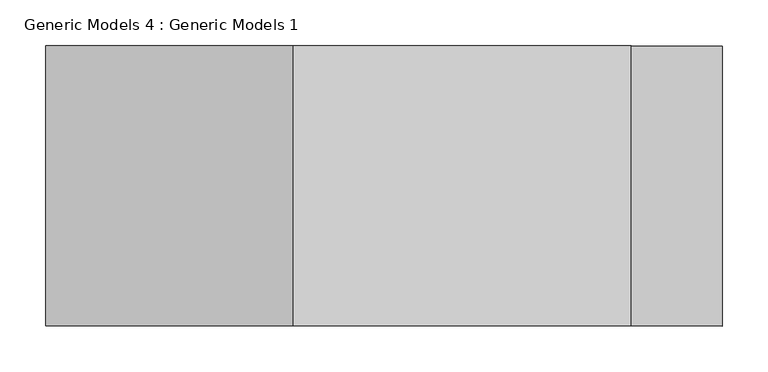
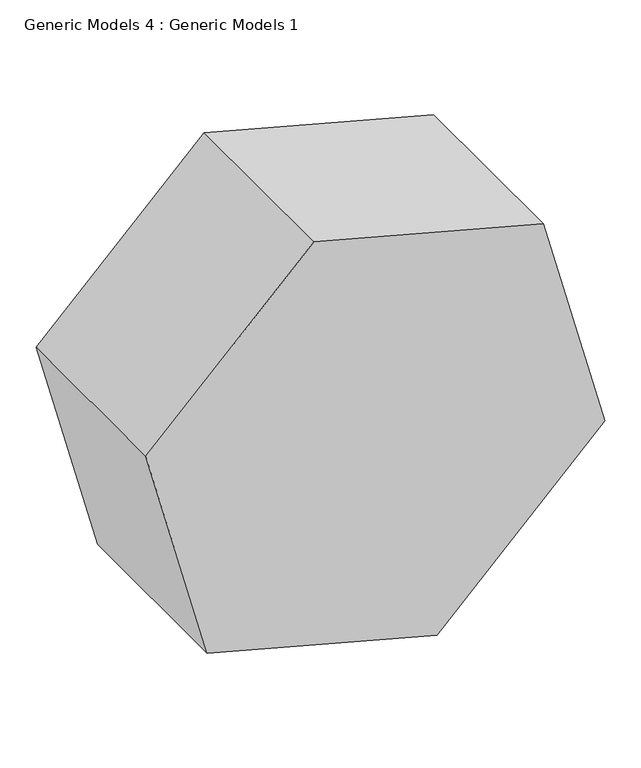
"""IFC4 building model written with IfcOpenShell, lengths in millimetres: proxy geometry, Generic Models 4 : Generic Models 1."""

from ifc_helpers import new_model, si_unit, frame, origin, place, context, project, spatial, polyline, outline, extrude, source, transform, mapped, element, save


def generic_models_4_generic_models_1_1de10410(model_context):
    return source(origin(), model_context, "Body", "SweptSolid", [
        extrude(outline(polyline([(904.7566299, -7206.2070438), (1003.366686, -7574.2247836), (733.9590024, -7843.6324672), (365.9412626, -7745.022411), (267.3312064, -7377.0046712), (536.73889, -7107.5969876), (904.7566299, -7206.2070438)])), frame((0.0, -9086.6225464, 0.0), z_axis=(0.0, 1.0, 0.0), x_axis=(0.0, 0.0, 1.0)), (0.0, 0.0, 1.0), 304.8),
    ])


if __name__ == "__main__":
    model = new_model("IFC4")
    model_context = context("Model", 3, world=origin())
    ifc_project = project(units=[si_unit("LENGTHUNIT", "METRE", prefix="MILLI")], contexts=[model_context])
    site = spatial("IfcSite", under=ifc_project)
    building = spatial("IfcBuilding", under=site)
    placement = place(None, origin())
    generic_models_4_generic_models_1_shape = generic_models_4_generic_models_1_1de10410(model_context)
    element("IfcBuildingElementProxy", 1, Name="Generic Models 4 : Generic Models 1", ObjectType="Generic Models 4 : Generic Models 1", at=placement, inside=building, context=model_context, shape_type="MappedRepresentation", body=[
        mapped(generic_models_4_generic_models_1_shape, transform((0.0, 0.0, 0.0), x_axis=(1.0, 0.0, 0.0), y_axis=(0.0, 1.0, 0.0), z_axis=(0.0, 0.0, 1.0))),
    ])
    save(model, "model.ifc")

# Revit data of these elements
# Element 1 (IfcBuildingElementProxy, "Generic Models 4 : Generic Models 1")
#   Materials on its faces: "Brick, Common"
# Materials
#   "Brick, Common": class "Masonry", colour RGB 170 98 104, transparency 0, Description = "Common brick", Cost = 0
